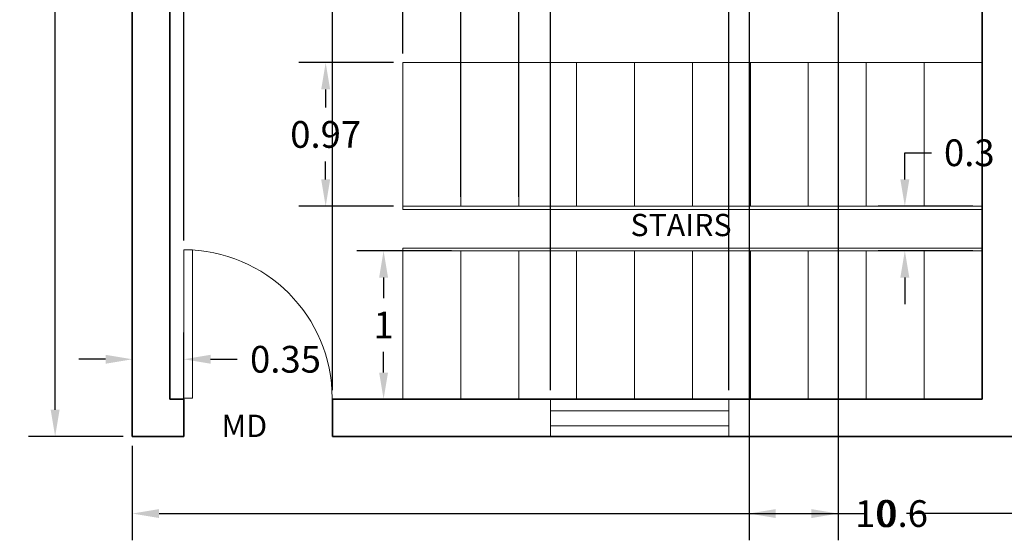
# Model space of a CAD drawing. Units: metres. Extents: x 1988.6 to 2001.1, y 2192 to 2202.5.
# Tile 1 of 6: x 1988.6 to 1995.3, y 2192 to 2195.5. Entities that reach past the tile are written whole.
import ezdxf

# ---------------------------------------------------------------- set-up
doc = ezdxf.new("R2010")
doc.units = ezdxf.units.M
for name, color, linetype, lineweight in [('A-ANNO-DIMS', 2, 'Continuous', 18), ('A-ANNO-TEXT', 7, 'Continuous', 18), ('A-AREA-IDEN', 7, 'Continuous', 18), ('A-DOOR', 3, 'Continuous', 18), ('A-FLOR-STRS', 7, 'Continuous', 18), ('A-GLAZ', 4, 'Continuous', 18), ('A-WALL', 7, 'Continuous', 35)]:
    doc.layers.add(name, color=color, linetype=linetype, lineweight=lineweight)
doc.styles.get("Standard").update_dxf_attribs({"font": 'arial.ttf'})
doc.dimstyles.get("Standard").update_dxf_attribs({"dimtxt": 0.18, "dimasz": 0.18, "dimexe": 0.18, "dimexo": 0.0625, "dimgap": 0.09, "dimtad": 0, "dimtih": 1, "dimtoh": 1, "dimdec": 4, "dimzin": 0, "dimdsep": 46, "dimtxsty": 'Standard', "dimcen": 0.09, "dimadec": 0, "dimazin": 0, "dimtfac": 1, "dimtdec": 4, "dimtofl": 0, "dimtmove": 0, "dimatfit": 3, "dimfxl": 1, "dimtolj": 1, "dimtzin": 0, "dimarcsym": 0})

# ---------------------------------------------------------------- blocks, each defined once
blk = doc.blocks.new('*U15')
for p, q in [((0, 0), (0, -100)), ((750, 0), (750, -100))]:
    blk.add_line(p, q)
blk.add_lwpolyline([(0, 0), (0, 750), (43.75, 750), (43.75, 0)], close=True)
blk.add_arc((0, 0), 750, 0, 90)
blk = doc.blocks.new('*D52')
at = {"layer": 'A-ANNO-DIMS', "color": 0, "lineweight": -2, "transparency": 16777216}
for p, q in [((1989.3818, 2192.6413), (1989.3818, 2192.0043)), ((1999.3818, 2192.6413), (1999.3818, 2192.0043)), ((1989.5618, 2192.1843), (1994.1717, 2192.1843)), ((1999.2018, 2192.1843), (1994.592, 2192.1843))]:
    blk.add_line(p, q, dxfattribs=at)
at = {"layer": 'A-ANNO-DIMS', "color": 0, "transparency": 16777216}
for points in [[(1989.5618, 2192.2143), (1989.5618, 2192.1543), (1989.3818, 2192.1843)], [(1999.2018, 2192.2143), (1999.2018, 2192.1543), (1999.3818, 2192.1843)]]:
    blk.add_solid(points, dxfattribs=at)
at = {"layer": 'Defpoints', "color": 0, "transparency": 16777216}
for p in [(1989.3818, 2192.7038), (1999.3818, 2192.7038), (1999.3818, 2192.1843)]:
    blk.add_point(p, dxfattribs=at)
at = {"layer": 'A-ANNO-DIMS', "color": 0, "transparency": 16777216, "insert": (1994.3818, 2192.1843), "char_height": 0.18, "attachment_point": 5}
blk.add_mtext('\\A1;10', dxfattribs=at)
blk = doc.blocks.new('*D53')
at = {"layer": 'A-ANNO-DIMS', "color": 0, "lineweight": -2, "transparency": 16777216}
for p, q in [((1989.3193, 2201.7538), (1988.6823, 2201.7538)), ((1988.8623, 2201.5738), (1988.8623, 2197.4107)), ((1988.8623, 2192.8838), (1988.8623, 2197.0469)), ((1989.3193, 2192.7038), (1988.6823, 2192.7038))]:
    blk.add_line(p, q, dxfattribs=at)
at = {"layer": 'A-ANNO-DIMS', "color": 0, "transparency": 16777216}
for points in [[(1988.8323, 2201.5738), (1988.8923, 2201.5738), (1988.8623, 2201.7538)], [(1988.8323, 2192.8838), (1988.8923, 2192.8838), (1988.8623, 2192.7038)]]:
    blk.add_solid(points, dxfattribs=at)
at = {"layer": 'Defpoints', "color": 0, "transparency": 16777216}
for p in [(1988.8623, 2201.7538), (1989.3818, 2201.7538), (1989.3818, 2192.7038)]:
    blk.add_point(p, dxfattribs=at)
at = {"layer": 'A-ANNO-DIMS', "color": 0, "transparency": 16777216, "insert": (1988.8623, 2197.2288), "char_height": 0.18, "attachment_point": 5}
blk.add_mtext('\\A1;9.05', dxfattribs=at)
blk = doc.blocks.new('*D58')
at = {"layer": 'A-ANNO-DIMS', "color": 0, "lineweight": -2, "transparency": 16777216}
for p, q in [((1989.3818, 2192.7663), (1989.3818, 2193.4033)), ((1989.7282, 2192.7663), (1989.7282, 2193.4033)), ((1989.2018, 2193.2233), (1989.0218, 2193.2233)), ((1989.9082, 2193.2233), (1990.0882, 2193.2233))]:
    blk.add_line(p, q, dxfattribs=at)
at = {"layer": 'A-ANNO-DIMS', "color": 0, "transparency": 16777216}
for points in [[(1989.2018, 2193.2533), (1989.2018, 2193.1933), (1989.3818, 2193.2233)], [(1989.9082, 2193.2533), (1989.9082, 2193.1933), (1989.7282, 2193.2233)]]:
    blk.add_solid(points, dxfattribs=at)
at = {"layer": 'Defpoints', "color": 0, "transparency": 16777216}
for p in [(1989.7282, 2193.2233), (1989.3818, 2192.7038), (1989.7282, 2192.7038)]:
    blk.add_point(p, dxfattribs=at)
at = {"layer": 'A-ANNO-DIMS', "color": 0, "transparency": 16777216, "insert": (1990.4127, 2193.2233), "char_height": 0.18, "attachment_point": 5}
blk.add_mtext('\\A1;0.35', dxfattribs=at)
blk = doc.blocks.new('*D59')
at = {"layer": 'A-ANNO-DIMS', "color": 0, "lineweight": -2, "transparency": 16777216}
for p, q in [((1989.7282, 2194.023), (1989.7282, 2202.4533)), ((1990.7282, 2193.0163), (1990.7282, 2202.4533)), ((1989.9082, 2202.2733), (1990.1051, 2202.2733)), ((1990.5482, 2202.2733), (1990.3514, 2202.2733))]:
    blk.add_line(p, q, dxfattribs=at)
at = {"layer": 'A-ANNO-DIMS', "color": 0, "transparency": 16777216}
for points in [[(1989.9082, 2202.3033), (1989.9082, 2202.2433), (1989.7282, 2202.2733)], [(1990.5482, 2202.3033), (1990.5482, 2202.2433), (1990.7282, 2202.2733)]]:
    blk.add_solid(points, dxfattribs=at)
at = {"layer": 'Defpoints', "color": 0, "transparency": 16777216}
for p in [(1990.7282, 2202.2733), (1989.7282, 2193.9605), (1990.7282, 2192.9538)]:
    blk.add_point(p, dxfattribs=at)
at = {"layer": 'A-ANNO-DIMS', "color": 0, "transparency": 16777216, "insert": (1990.2282, 2202.2733), "char_height": 0.18, "attachment_point": 5}
blk.add_mtext('\\A1;1', dxfattribs=at)
blk = doc.blocks.new('*D60')
at = {"layer": 'A-ANNO-DIMS', "color": 0, "lineweight": -2, "transparency": 16777216}
for p, q in [((1990.7282, 2193.0163), (1990.7282, 2202.4533)), ((1992.1958, 2193.0163), (1992.1958, 2202.4533)), ((1990.9082, 2202.2733), (1991.1467, 2202.2733)), ((1992.0158, 2202.2733), (1991.7773, 2202.2733))]:
    blk.add_line(p, q, dxfattribs=at)
at = {"layer": 'A-ANNO-DIMS', "color": 0, "transparency": 16777216}
for points in [[(1990.9082, 2202.3033), (1990.9082, 2202.2433), (1990.7282, 2202.2733)], [(1992.0158, 2202.3033), (1992.0158, 2202.2433), (1992.1958, 2202.2733)]]:
    blk.add_solid(points, dxfattribs=at)
at = {"layer": 'Defpoints', "color": 0, "transparency": 16777216}
for p in [(1992.1958, 2202.2733), (1990.7282, 2192.9538), (1992.1958, 2192.9538)]:
    blk.add_point(p, dxfattribs=at)
at = {"layer": 'A-ANNO-DIMS', "color": 0, "transparency": 16777216, "insert": (1991.462, 2202.2733), "char_height": 0.18, "attachment_point": 5}
blk.add_mtext('\\A1;1.47', dxfattribs=at)
blk = doc.blocks.new('*D61')
at = {"layer": 'A-ANNO-DIMS', "color": 0, "lineweight": -2, "transparency": 16777216}
for p, q in [((1992.1958, 2193.0163), (1992.1958, 2202.4533)), ((1993.3958, 2193.0163), (1993.3958, 2202.4533)), ((1992.3758, 2202.2733), (1992.5513, 2202.2733)), ((1993.2158, 2202.2733), (1993.0402, 2202.2733))]:
    blk.add_line(p, q, dxfattribs=at)
at = {"layer": 'A-ANNO-DIMS', "color": 0, "transparency": 16777216}
for points in [[(1992.3758, 2202.3033), (1992.3758, 2202.2433), (1992.1958, 2202.2733)], [(1993.2158, 2202.3033), (1993.2158, 2202.2433), (1993.3958, 2202.2733)]]:
    blk.add_solid(points, dxfattribs=at)
at = {"layer": 'Defpoints', "color": 0, "transparency": 16777216}
for p in [(1993.3958, 2202.2733), (1992.1958, 2192.9538), (1993.3958, 2192.9538)]:
    blk.add_point(p, dxfattribs=at)
at = {"layer": 'A-ANNO-DIMS', "color": 0, "transparency": 16777216, "insert": (1992.7958, 2202.2733), "char_height": 0.18, "attachment_point": 5}
blk.add_mtext('\\A1;1.2', dxfattribs=at)
blk = doc.blocks.new('*D62')
at = {"layer": 'A-ANNO-DIMS', "color": 0, "lineweight": -2, "transparency": 16777216}
for p, q in [((1989.6351, 2193.0163), (1989.6351, 2202.4533)), ((1991.2026, 2195.283), (1991.2026, 2202.4533)), ((1989.8151, 2202.2733), (1990.1035, 2202.2733)), ((1991.0226, 2202.2733), (1990.7342, 2202.2733))]:
    blk.add_line(p, q, dxfattribs=at)
at = {"layer": 'A-ANNO-DIMS', "color": 0, "transparency": 16777216}
for points in [[(1989.8151, 2202.3033), (1989.8151, 2202.2433), (1989.6351, 2202.2733)], [(1991.0226, 2202.3033), (1991.0226, 2202.2433), (1991.2026, 2202.2733)]]:
    blk.add_solid(points, dxfattribs=at)
at = {"layer": 'Defpoints', "color": 0, "transparency": 16777216}
for p in [(1991.2026, 2202.2733), (1991.2026, 2195.2205), (1989.6351, 2192.9538)]:
    blk.add_point(p, dxfattribs=at)
at = {"layer": 'A-ANNO-DIMS', "color": 0, "transparency": 16777216, "insert": (1990.4189, 2202.2733), "char_height": 0.18, "attachment_point": 5}
blk.add_mtext('\\A1;1.57', dxfattribs=at)
blk = doc.blocks.new('*D63')
at = {"layer": 'A-ANNO-DIMS', "color": 0, "lineweight": -2, "transparency": 16777216}
for p, q in [((1991.2026, 2195.283), (1991.2026, 2202.4533)), ((1995.1007, 2195.283), (1995.1007, 2202.4533)), ((1991.3826, 2202.2733), (1992.7578, 2202.2733)), ((1994.9207, 2202.2733), (1993.5455, 2202.2733))]:
    blk.add_line(p, q, dxfattribs=at)
at = {"layer": 'A-ANNO-DIMS', "color": 0, "transparency": 16777216}
for points in [[(1991.3826, 2202.3033), (1991.3826, 2202.2433), (1991.2026, 2202.2733)], [(1994.9207, 2202.3033), (1994.9207, 2202.2433), (1995.1007, 2202.2733)]]:
    blk.add_solid(points, dxfattribs=at)
at = {"layer": 'Defpoints', "color": 0, "transparency": 16777216}
for p in [(1995.1007, 2202.2733), (1991.2026, 2195.2205), (1995.1007, 2195.2205)]:
    blk.add_point(p, dxfattribs=at)
at = {"layer": 'A-ANNO-DIMS', "color": 0, "transparency": 16777216, "insert": (1993.1516, 2202.2733), "char_height": 0.18, "attachment_point": 5}
blk.add_mtext('\\A1;3.898', dxfattribs=at)
blk = doc.blocks.new('*D64')
at = {"layer": 'A-ANNO-DIMS', "color": 0, "lineweight": -2, "transparency": 16777216}
for p, q in [((1991.1401, 2195.2205), (1990.5031, 2195.2205)), ((1990.6831, 2195.0405), (1990.6831, 2194.919)), ((1990.6831, 2194.4338), (1990.6831, 2194.5552)), ((1991.1401, 2194.2538), (1990.5031, 2194.2538))]:
    blk.add_line(p, q, dxfattribs=at)
at = {"layer": 'A-ANNO-DIMS', "color": 0, "transparency": 16777216}
for points in [[(1990.6531, 2195.0405), (1990.7131, 2195.0405), (1990.6831, 2195.2205)], [(1990.6531, 2194.4338), (1990.7131, 2194.4338), (1990.6831, 2194.2538)]]:
    blk.add_solid(points, dxfattribs=at)
at = {"layer": 'Defpoints', "color": 0, "transparency": 16777216}
for p in [(1990.6831, 2195.2205), (1991.2026, 2195.2205), (1991.2026, 2194.2538)]:
    blk.add_point(p, dxfattribs=at)
at = {"layer": 'A-ANNO-DIMS', "color": 0, "transparency": 16777216, "insert": (1990.6831, 2194.7371), "char_height": 0.18, "attachment_point": 5}
blk.add_mtext('\\A1;0.97', dxfattribs=at)
blk = doc.blocks.new('*D65')
at = {"layer": 'A-ANNO-DIMS', "color": 0, "lineweight": -2, "transparency": 16777216}
for p, q in [((1991.5299, 2193.9538), (1990.8929, 2193.9538)), ((1991.0729, 2193.7738), (1991.0729, 2193.6341)), ((1991.0729, 2193.1338), (1991.0729, 2193.2734)), ((1991.5299, 2192.9538), (1990.8929, 2192.9538))]:
    blk.add_line(p, q, dxfattribs=at)
at = {"layer": 'A-ANNO-DIMS', "color": 0, "transparency": 16777216}
for points in [[(1991.0429, 2193.7738), (1991.1029, 2193.7738), (1991.0729, 2193.9538)], [(1991.0429, 2193.1338), (1991.1029, 2193.1338), (1991.0729, 2192.9538)]]:
    blk.add_solid(points, dxfattribs=at)
at = {"layer": 'Defpoints', "color": 0, "transparency": 16777216}
for p in [(1991.0729, 2193.9538), (1991.5924, 2193.9538), (1991.5924, 2192.9538)]:
    blk.add_point(p, dxfattribs=at)
at = {"layer": 'A-ANNO-DIMS', "color": 0, "transparency": 16777216, "insert": (1991.0729, 2193.4538), "char_height": 0.18, "attachment_point": 5}
blk.add_mtext('\\A1;1', dxfattribs=at)
blk = doc.blocks.new('*D66')
at = {"layer": 'A-ANNO-DIMS', "color": 0, "lineweight": -2, "transparency": 16777216}
for p, q in [((1994.5812, 2194.4338), (1994.5812, 2194.6138)), ((1994.5812, 2194.6138), (1994.7612, 2194.6138)), ((1995.0382, 2194.2538), (1994.4012, 2194.2538)), ((1995.0382, 2193.9538), (1994.4012, 2193.9538)), ((1994.5812, 2193.7738), (1994.5812, 2193.5938))]:
    blk.add_line(p, q, dxfattribs=at)
at = {"layer": 'A-ANNO-DIMS', "color": 0, "transparency": 16777216}
for points in [[(1994.5512, 2194.4338), (1994.6112, 2194.4338), (1994.5812, 2194.2538)], [(1994.5512, 2193.7738), (1994.6112, 2193.7738), (1994.5812, 2193.9538)]]:
    blk.add_solid(points, dxfattribs=at)
at = {"layer": 'Defpoints', "color": 0, "transparency": 16777216}
for p in [(1994.5812, 2194.2538), (1995.1007, 2194.2538), (1995.1007, 2193.9538)]:
    blk.add_point(p, dxfattribs=at)
at = {"layer": 'A-ANNO-DIMS', "color": 0, "transparency": 16777216, "insert": (1995.015, 2194.6138), "char_height": 0.18, "attachment_point": 5}
blk.add_mtext('\\A1;0.3', dxfattribs=at)
blk = doc.blocks.new('*D67')
at = {"layer": 'A-ANNO-DIMS', "color": 0, "lineweight": -2, "transparency": 16777216}
for p, q in [((1991.5924, 2194.3163), (1991.5924, 2202.4533)), ((1991.9822, 2194.3163), (1991.9822, 2202.4533)), ((1991.4124, 2202.2733), (1991.2324, 2202.2733)), ((1992.1622, 2202.2733), (1992.3422, 2202.2733))]:
    blk.add_line(p, q, dxfattribs=at)
at = {"layer": 'A-ANNO-DIMS', "color": 0, "transparency": 16777216}
for points in [[(1991.4124, 2202.3033), (1991.4124, 2202.2433), (1991.5924, 2202.2733)], [(1992.1622, 2202.3033), (1992.1622, 2202.2433), (1991.9822, 2202.2733)]]:
    blk.add_solid(points, dxfattribs=at)
at = {"layer": 'Defpoints', "color": 0, "transparency": 16777216}
for p in [(1991.9822, 2202.2733), (1991.5924, 2194.2538), (1991.9822, 2194.2538)]:
    blk.add_point(p, dxfattribs=at)
at = {"layer": 'A-ANNO-DIMS', "color": 0, "transparency": 16777216, "insert": (1992.6662, 2202.2733), "char_height": 0.18, "attachment_point": 5}
blk.add_mtext('\\A1;0.39', dxfattribs=at)
blk = doc.blocks.new('*D73')
at = {"layer": 'A-ANNO-DIMS', "color": 0, "lineweight": -2, "transparency": 16777216}
for p, q in [((1993.5324, 2199.3495), (1993.5324, 2192.0043)), ((1994.1324, 2199.3495), (1994.1324, 2192.0043)), ((1993.7124, 2192.1843), (1993.9524, 2192.1843)), ((1994.1324, 2192.1843), (1994.3124, 2192.1843))]:
    blk.add_line(p, q, dxfattribs=at)
at = {"layer": 'A-ANNO-DIMS', "color": 0, "transparency": 16777216}
for points in [[(1993.7124, 2192.2143), (1993.7124, 2192.1543), (1993.5324, 2192.1843)], [(1993.9524, 2192.2143), (1993.9524, 2192.1543), (1994.1324, 2192.1843)]]:
    blk.add_solid(points, dxfattribs=at)
at = {"layer": 'Defpoints', "color": 0, "transparency": 16777216}
for p in [(1993.5324, 2199.412), (1994.1324, 2199.412), (1994.1324, 2192.1843)]:
    blk.add_point(p, dxfattribs=at)
at = {"layer": 'A-ANNO-DIMS', "color": 0, "transparency": 16777216, "insert": (1994.5662, 2192.1843), "char_height": 0.18, "attachment_point": 5}
blk.add_mtext('\\A1;0.6', dxfattribs=at)

msp = doc.modelspace()

# ---------------------------------------------------------------- linework, layer by layer
at = {"layer": 'A-FLOR-STRS'}
for p, q in [((1991.2026, 2194.2538), (1991.2026, 2195.2205)), ((1991.2026, 2195.2205), (1995.1007, 2195.2205)), ((1991.5924, 2194.2538), (1991.5924, 2195.2205)), ((1991.9822, 2194.2538), (1991.9822, 2195.2205)), ((1992.372, 2194.2538), (1992.372, 2195.2205)), ((1992.7618, 2194.2538), (1992.7618, 2195.2205)), ((1993.1516, 2194.2538), (1993.1516, 2195.2205)), ((1993.5414, 2194.2538), (1993.5414, 2195.2205)), ((1993.9313, 2194.2538), (1993.9313, 2195.2205)), ((1994.3211, 2194.2538), (1994.3211, 2195.2205)), ((1994.7109, 2194.2538), (1994.7109, 2195.2205)), ((1991.2026, 2194.2538), (1995.1007, 2194.2538)), ((1991.2026, 2194.2326), (1991.2026, 2194.2538)), ((1995.1007, 2194.2326), (1991.2026, 2194.2326)), ((1995.1007, 2193.9703), (1991.2026, 2193.9703)), ((1991.2026, 2193.9703), (1991.2026, 2193.9538)), ((1991.2026, 2193.9538), (1995.1007, 2193.9538)), ((1991.2026, 2193.9538), (1991.2026, 2192.9538)), ((1991.5924, 2193.9538), (1991.5924, 2192.9538)), ((1991.9822, 2193.9538), (1991.9822, 2192.9538)), ((1992.372, 2193.9538), (1992.372, 2192.9538)), ((1992.7618, 2193.9538), (1992.7618, 2192.9538)), ((1993.1516, 2193.9538), (1993.1516, 2192.9538)), ((1993.5414, 2193.9538), (1993.5414, 2192.9538)), ((1993.9313, 2193.9538), (1993.9313, 2192.9538)), ((1994.3211, 2193.9538), (1994.3211, 2192.9538)), ((1994.7109, 2193.9538), (1994.7109, 2192.9538))]:
    msp.add_line(p, q, dxfattribs=at)
at = {"layer": 'A-GLAZ'}
for p, q in [((1992.1958, 2192.9538), (1993.3958, 2192.9538)), ((1992.1958, 2192.7038), (1992.1958, 2192.9538)), ((1993.3958, 2192.9538), (1993.3958, 2192.7038)), ((1992.1958, 2192.8755), (1993.3958, 2192.8755)), ((1992.1958, 2192.7762), (1993.3958, 2192.7762)), ((1992.1958, 2192.7038), (1993.3958, 2192.7038))]:
    msp.add_line(p, q, dxfattribs=at)
at = {"layer": 'A-WALL'}
for p, q in [((1989.3818, 2201.7538), (1989.3818, 2192.7038)), ((1989.6351, 2198.2651), (1989.6351, 2192.9538)), ((1995.1007, 2192.9538), (1995.1007, 2196.7854)), ((1989.6351, 2192.9538), (1989.7282, 2192.9538)), ((1989.7282, 2192.9538), (1989.7282, 2192.7038)), ((1990.7282, 2192.9538), (1990.7282, 2192.7038)), ((1990.7282, 2192.9538), (1995.1007, 2192.9538)), ((1989.3818, 2192.7038), (1989.7282, 2192.7038)), ((1990.7282, 2192.7038), (1999.3818, 2192.7038))]:
    msp.add_line(p, q, dxfattribs=at)

# ---------------------------------------------------------------- block references
at = {"layer": 'A-DOOR', "xscale": 0.0013314374781155, "yscale": 0.0013314374781155, "zscale": 0.0013314374781155}
msp.add_blockref('*U15', (1989.7282, 2192.9619), dxfattribs=at)

# ---------------------------------------------------------------- texts
at = {"layer": 'A-ANNO-TEXT', "insert": (1989.9822, 2192.85), "char_height": 0.15, "attachment_point": 1}
msp.add_mtext_dynamic_manual_height_columns('MD ', width=0.386628, gutter_width=12.5, heights=[0], dxfattribs=at)
at = {"layer": 'A-AREA-IDEN', "insert": (1992.7344, 2194.2023), "char_height": 0.15, "attachment_point": 1}
msp.add_mtext_dynamic_manual_height_columns('STAIRS ', width=0.386628, gutter_width=12.5, heights=[0], dxfattribs=at)

# ---------------------------------------------------------------- dimensions: what is measured, and where the dimension line sits
at = {"layer": 'A-ANNO-DIMS'}
for base, p1, p2, override, picture, middle in [((1991.2026, 2202.2733), (1989.6351, 2192.9538), (1991.2026, 2195.2205), {"dimdec": 2, "dimlfac": 1, "dimrnd": 0, "dimzin": 0, "dimdsep": 46, "dimlunit": 2}, '*D62', (1990.4189, 2202.2733)), ((1990.7282, 2202.2733), (1989.7282, 2193.9605), (1990.7282, 2192.9538), {"dimdec": 0, "dimlfac": 1, "dimrnd": 0, "dimzin": 0, "dimdsep": 46, "dimlunit": 2}, '*D59', (1990.2282, 2202.2733)), ((1992.1958, 2202.2733), (1990.7282, 2192.9538), (1992.1958, 2192.9538), {"dimdec": 2, "dimlfac": 1, "dimrnd": 0, "dimzin": 0, "dimdsep": 46, "dimlunit": 2}, '*D60', (1991.462, 2202.2733)), ((1995.1007, 2202.2733), (1991.2026, 2195.2205), (1995.1007, 2195.2205), {"dimdec": 3, "dimlfac": 1, "dimrnd": 0, "dimzin": 0, "dimdsep": 46, "dimlunit": 2}, '*D63', (1993.1516, 2202.2733)), ((1991.9822, 2202.2733), (1991.5924, 2194.2538), (1991.9822, 2194.2538), {"dimdec": 2, "dimlfac": 1, "dimrnd": 0, "dimzin": 0, "dimdsep": 46, "dimlunit": 2}, '*D67', (1992.6662, 2202.2733)), ((1993.3958, 2202.2733), (1992.1958, 2192.9538), (1993.3958, 2192.9538), {"dimdec": 1, "dimlfac": 1, "dimrnd": 0, "dimzin": 0, "dimdsep": 46, "dimlunit": 2}, '*D61', (1992.7958, 2202.2733)), ((1994.1324, 2192.1843), (1993.5324, 2199.412), (1994.1324, 2199.412), {"dimdec": 1, "dimlfac": 1, "dimrnd": 0, "dimzin": 0, "dimdsep": 46, "dimlunit": 2}, '*D73', (1994.5662, 2192.1843)), ((1989.7282, 2193.2233), (1989.3818, 2192.7038), (1989.7282, 2192.7038), {"dimdec": 2, "dimlfac": 1, "dimrnd": 0, "dimzin": 0, "dimdsep": 46, "dimlunit": 2}, '*D58', (1990.4127, 2193.2233)), ((1999.3818, 2192.1843), (1989.3818, 2192.7038), (1999.3818, 2192.7038), {"dimdec": 0, "dimlfac": 1, "dimrnd": 0, "dimzin": 0, "dimdsep": 46, "dimlunit": 2}, '*D52', (1994.3818, 2192.1843))]:
    dim = msp.add_linear_dim(base=base, p1=p1, p2=p2, dimstyle='Standard', override=override, dxfattribs=at)
    dim.commit()
    dim.dimension.update_dxf_attribs({"geometry": picture, "text_midpoint": middle})
for base, p1, p2, override, picture, middle in [((1988.8623, 2201.7538), (1989.3818, 2192.7038), (1989.3818, 2201.7538), {"dimdec": 2, "dimlfac": 1, "dimrnd": 0, "dimzin": 0, "dimdsep": 46, "dimlunit": 2}, '*D53', (1988.8623, 2197.2288)), ((1990.6831, 2195.2205), (1991.2026, 2194.2538), (1991.2026, 2195.2205), {"dimdec": 2, "dimlfac": 1, "dimrnd": 0, "dimzin": 0, "dimdsep": 46, "dimlunit": 2}, '*D64', (1990.6831, 2194.7371)), ((1994.5812, 2194.2538), (1995.1007, 2193.9538), (1995.1007, 2194.2538), {"dimdec": 1, "dimlfac": 1, "dimrnd": 0, "dimzin": 0, "dimdsep": 46, "dimlunit": 2}, '*D66', (1995.015, 2194.6138)), ((1991.0729, 2193.9538), (1991.5924, 2192.9538), (1991.5924, 2193.9538), {"dimdec": 0, "dimlfac": 1, "dimrnd": 0, "dimzin": 0, "dimdsep": 46, "dimlunit": 2}, '*D65', (1991.0729, 2193.4538))]:
    dim = msp.add_linear_dim(base=base, p1=p1, p2=p2, angle=90, dimstyle='Standard', override=override, dxfattribs=at)
    dim.commit()
    dim.dimension.update_dxf_attribs({"geometry": picture, "text_midpoint": middle})

doc.saveas('drawing.dxf')
